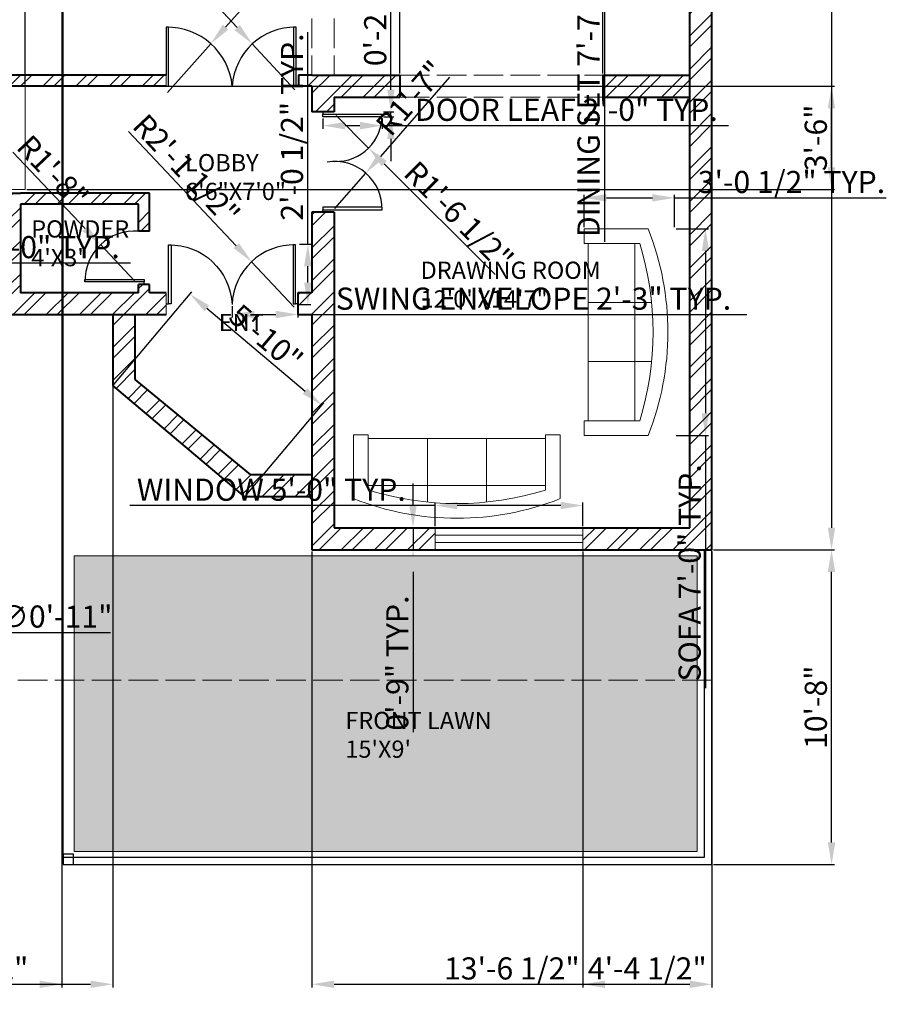
# Model space of a CAD drawing. Units: inches. Extents: x 3815 to 4442, y 1449 to 2534.
# Tile 2 of 5: x 4090 to 4442, y 1449 to 1850. Entities that reach past the tile are written whole.
import ezdxf

# ---------------------------------------------------------------- set-up
doc = ezdxf.new("R2010")
doc.units = ezdxf.units.IN
doc.linetypes.add('ACAD_ISO02W100', pattern=[15, 12, -3])
for name, color, linetype, lineweight in [('A-ANNO-DIMS', 2, 'Continuous', 18), ('A-AREA-IDEN', 7, 'Continuous', 20), ('A-DOOR', 4, 'Continuous', 25), ('A-FLOR-STRS', 7, 'Continuous', 20), ('A-FURN', 8, 'Continuous', 18), ('A-GLAZ', 4, 'Continuous', 20), ('A-ROOF-OVHD', 8, 'ACAD_ISO02W100', 13), ('A-WALL', 7, 'Continuous', 40), ('A-WALL-OVHD', 8, 'ACAD_ISO02W100', 18), ('A-WALL-PATT', 8, 'Continuous', 13), ('C-PROP', 7, 'Continuous', 30), ('L-PLNT', 3, 'Continuous', 18), ('L-PLNT-PATT', 9, 'Continuous', 13)]:
    doc.layers.add(name, color=color, linetype=linetype, lineweight=lineweight)
doc.styles.get("Standard").update_dxf_attribs({"font": 'arial.ttf'})
doc.dimstyles.new('ISO-25', dxfattribs={"dimtxt": 9, "dimasz": 9, "dimexe": 1.25, "dimexo": 0.625, "dimtad": 1, "dimdec": 1, "dimrnd": 9, "dimlunit": 3, "dimtxsty": 'Standard', "dimcen": 2.5, "dimadec": 0, "dimazin": 0, "dimtfac": 1, "dimtdec": 1, "dimtmove": 0, "dimatfit": 3, "dimfxl": 1, "dimarcsym": 0})

# ---------------------------------------------------------------- blocks, each defined once
blk = doc.blocks.new('Sofa - Roundback 7 ft.')
for p, q in [((-12.00002, -32.4421), (-12.00003, -6.5971)), ((11.99997, -32.4421), (11.99998, -6.5971)), ((-36.000027, -34), (-36.000027, -11.4696)), ((35.99998, -34), (35.99998, -11.4696)), ((-35.999844, -13.3819), (35.9998, -13.3819)), ((-36.000027, -32.4421), (35.99998, -32.4421))]:
    blk.add_line(p, q)
for points in [[(-36.000027, -34), (-42.000027, -34), (-42.000027, -8)], [(41.99998, -8), (41.99998, -34), (35.99998, -34)]]:
    blk.add_lwpolyline(points)
for centre, radius, start, end in [((0, -114.25), 114.25, 68.43141, 111.5686), ((-0.00001, -127.1968), 121.1968, 72.72033, 107.2797)]:
    blk.add_arc(centre, radius, start, end)
blk = doc.blocks.new('WIN-W60-9IN')
for p, q in [((0, 9), (0, 0)), ((60, 9), (60, 0)), ((60, 6), (0, 6)), ((60, 3), (0, 3))]:
    blk.add_line(p, q)
blk = doc.blocks.new('DOOR-SWING-24IN')
for p, q in [((25.78, 24.32), (24.78, 24.32)), ((24.78, 24.32), (24.78, 0.32)), ((25.78, 0.32), (25.78, 24.32)), ((24.78, 0.32), (25.78, 0.32)), ((26.78, 0.32), (25.78, 0.32))]:
    blk.add_line(p, q)
blk.add_arc((25.28, -0.98), 25.3, 88.8677, 177.7775)
blk = doc.blocks.new('DOOR-LEAF-24IN')
for p, q in [((0, 2), (0, 1)), ((0, 1), (24, 1)), ((0, 0), (0, 1)), ((24, 0), (0, 0)), ((24, 1), (24, 0))]:
    blk.add_line(p, q)
blk = doc.blocks.new('SITE-PIER')
blk.add_lwpolyline([(0, 0), (4.2, 0), (4.2, 4.28), (0, 4.28)], close=True)
blk = doc.blocks.new('*D18')
at = {"layer": 'A-ANNO-DIMS', "color": 0, "lineweight": -2, "transparency": 16777216}
for p, q in [((4356.58, 1764.74), (4369.81, 1764.74)), ((4368.56, 1755.74), (4368.56, 1689.74)), ((4356.58, 1680.74), (4369.81, 1680.74)), ((4368.56, 1680.74), (4368.56, 1577.95))]:
    blk.add_line(p, q, dxfattribs=at)
at = {"layer": 'A-ANNO-DIMS', "color": 0, "lineweight": 100, "transparency": 16777216}
for points in [[(4367.06, 1755.74), (4370.06, 1755.74), (4368.56, 1764.74)], [(4367.06, 1689.74), (4370.06, 1689.74), (4368.56, 1680.74)]]:
    blk.add_solid(points, dxfattribs=at)
at = {"layer": 'Defpoints', "color": 0, "lineweight": 100, "transparency": 16777216}
for p in [(4355.96, 1764.74), (4355.96, 1680.74), (4368.56, 1680.74)]:
    blk.add_point(p, dxfattribs=at)
at = {"layer": 'A-ANNO-DIMS', "color": 0, "transparency": 16777216, "insert": (4363.28, 1624.85), "char_height": 9, "attachment_point": 5, "rotation": 90}
blk.add_mtext('SOFA 7\'-0" TYP.', dxfattribs=at)
blk = doc.blocks.new('*D19')
at = {"layer": 'A-ANNO-DIMS', "color": 0, "lineweight": -2, "transparency": 16777216}
for p, q in [((4319.29, 1765.37), (4319.29, 1778.59)), ((4355.96, 1765.37), (4355.96, 1778.59)), ((4328.29, 1777.34), (4346.96, 1777.34)), ((4355.96, 1777.34), (4442.03, 1777.34))]:
    blk.add_line(p, q, dxfattribs=at)
at = {"layer": 'A-ANNO-DIMS', "color": 0, "lineweight": 100, "transparency": 16777216}
for points in [[(4328.29, 1778.84), (4328.29, 1775.84), (4319.29, 1777.34)], [(4346.96, 1778.84), (4346.96, 1775.84), (4355.96, 1777.34)]]:
    blk.add_solid(points, dxfattribs=at)
at = {"layer": 'Defpoints', "color": 0, "lineweight": 100, "transparency": 16777216}
for p in [(4355.96, 1777.34), (4319.29, 1764.74), (4355.96, 1764.74)]:
    blk.add_point(p, dxfattribs=at)
at = {"layer": 'A-ANNO-DIMS', "color": 0, "transparency": 16777216, "insert": (4403.5, 1782.62), "char_height": 9, "attachment_point": 5}
blk.add_mtext('3\'-0 1/2" TYP.', dxfattribs=at)
blk = doc.blocks.new('*D20')
at = {"layer": 'A-ANNO-DIMS', "color": 0, "lineweight": -2, "transparency": 16777216}
for p, q in [((4213.13, 1809.67), (4213.13, 1805.45)), ((4237.13, 1809.67), (4237.13, 1805.45)), ((4222.13, 1806.7), (4228.13, 1806.7)), ((4237.13, 1806.7), (4377.94, 1806.7))]:
    blk.add_line(p, q, dxfattribs=at)
at = {"layer": 'A-ANNO-DIMS', "color": 0, "lineweight": 100, "transparency": 16777216}
for points in [[(4222.13, 1808.2), (4222.13, 1805.2), (4213.13, 1806.7)], [(4228.13, 1808.2), (4228.13, 1805.2), (4237.13, 1806.7)]]:
    blk.add_solid(points, dxfattribs=at)
at = {"layer": 'Defpoints', "color": 0, "lineweight": 100, "transparency": 16777216}
for p in [(4213.13, 1810.3), (4237.13, 1810.3), (4237.13, 1806.7)]:
    blk.add_point(p, dxfattribs=at)
at = {"layer": 'A-ANNO-DIMS', "color": 0, "transparency": 16777216, "insert": (4312.03, 1811.98), "char_height": 9, "attachment_point": 5}
blk.add_mtext('DOOR LEAF 2\'-0" TYP.', dxfattribs=at)
blk = doc.blocks.new('*D21')
at = {"layer": 'A-ANNO-DIMS', "color": 0, "lineweight": -2, "transparency": 16777216}
for p, q in [((4240.73, 1821.3), (4240.73, 1886.41)), ((4237.75, 1812.3), (4241.98, 1812.3)), ((4237.75, 1810.3), (4241.98, 1810.3)), ((4240.73, 1810.3), (4240.73, 1812.3)), ((4240.73, 1801.3), (4240.73, 1792.3))]:
    blk.add_line(p, q, dxfattribs=at)
at = {"layer": 'A-ANNO-DIMS', "color": 0, "lineweight": 100, "transparency": 16777216}
for points in [[(4239.23, 1821.3), (4242.23, 1821.3), (4240.73, 1812.3)], [(4239.23, 1801.3), (4242.23, 1801.3), (4240.73, 1810.3)]]:
    blk.add_solid(points, dxfattribs=at)
at = {"layer": 'Defpoints', "color": 0, "lineweight": 100, "transparency": 16777216}
for p in [(4237.13, 1812.3), (4237.13, 1810.3), (4240.73, 1812.3)]:
    blk.add_point(p, dxfattribs=at)
at = {"layer": 'A-ANNO-DIMS', "color": 0, "transparency": 16777216, "insert": (4235.51, 1858.35), "char_height": 9, "attachment_point": 5, "rotation": 90}
blk.add_mtext('0\'-2" TYP.', dxfattribs=at)
blk = doc.blocks.new('*D24')
at = {"layer": 'A-ANNO-DIMS', "color": 0, "lineweight": -2, "transparency": 16777216}
for p, q in [((4258.71, 1643.87), (4258.71, 1653.49)), ((4318.71, 1643.87), (4318.71, 1653.49)), ((4258.71, 1652.24), (4134.57, 1652.24)), ((4309.71, 1652.24), (4267.71, 1652.24))]:
    blk.add_line(p, q, dxfattribs=at)
at = {"layer": 'A-ANNO-DIMS', "color": 0, "lineweight": 100, "transparency": 16777216}
for points in [[(4267.71, 1653.74), (4267.71, 1650.74), (4258.71, 1652.24)], [(4309.71, 1653.74), (4309.71, 1650.74), (4318.71, 1652.24)]]:
    blk.add_solid(points, dxfattribs=at)
at = {"layer": 'Defpoints', "color": 0, "lineweight": 100, "transparency": 16777216}
for p in [(4258.71, 1652.24), (4258.71, 1643.24), (4318.71, 1643.24)]:
    blk.add_point(p, dxfattribs=at)
at = {"layer": 'A-ANNO-DIMS', "color": 0, "transparency": 16777216, "insert": (4192.14, 1657.52), "char_height": 9, "attachment_point": 5}
blk.add_mtext('WINDOW 5\'-0" TYP.', dxfattribs=at)
blk = doc.blocks.new('*D25')
at = {"layer": 'A-ANNO-DIMS', "color": 0, "lineweight": -2, "transparency": 16777216}
for p, q in [((4249.71, 1652.24), (4249.71, 1661.24)), ((4258.08, 1643.24), (4248.46, 1643.24)), ((4249.71, 1643.24), (4249.71, 1634.24)), ((4258.08, 1634.24), (4248.46, 1634.24)), ((4249.71, 1625.24), (4249.71, 1560.13))]:
    blk.add_line(p, q, dxfattribs=at)
at = {"layer": 'A-ANNO-DIMS', "color": 0, "lineweight": 100, "transparency": 16777216}
for points in [[(4248.21, 1652.24), (4251.21, 1652.24), (4249.71, 1643.24)], [(4248.21, 1625.24), (4251.21, 1625.24), (4249.71, 1634.24)]]:
    blk.add_solid(points, dxfattribs=at)
at = {"layer": 'Defpoints', "color": 0, "lineweight": 100, "transparency": 16777216}
for p in [(4258.71, 1643.24), (4249.71, 1634.24), (4258.71, 1634.24)]:
    blk.add_point(p, dxfattribs=at)
at = {"layer": 'A-ANNO-DIMS', "color": 0, "transparency": 16777216, "insert": (4244.49, 1588.19), "char_height": 9, "attachment_point": 5, "rotation": 90}
blk.add_mtext('0\'-9" TYP.', dxfattribs=at)
blk = doc.blocks.new('*D28')
at = {"layer": 'A-ANNO-DIMS', "color": 0, "lineweight": -2, "transparency": 16777216}
for p, q in [((3958.12, 1746.08), (3958.12, 1752.11)), ((3967.12, 1750.86), (3985.12, 1750.86)), ((3994.12, 1746.08), (3994.12, 1752.11)), ((3994.12, 1750.86), (4134.93, 1750.86))]:
    blk.add_line(p, q, dxfattribs=at)
at = {"layer": 'A-ANNO-DIMS', "color": 0, "lineweight": 100, "transparency": 16777216}
for points in [[(3967.12, 1752.36), (3967.12, 1749.36), (3958.12, 1750.86)], [(3985.12, 1752.36), (3985.12, 1749.36), (3994.12, 1750.86)]]:
    blk.add_solid(points, dxfattribs=at)
at = {"layer": 'Defpoints', "color": 0, "lineweight": 100, "transparency": 16777216}
for p in [(3994.12, 1750.86), (3958.12, 1745.46), (3994.12, 1745.46)]:
    blk.add_point(p, dxfattribs=at)
at = {"layer": 'A-ANNO-DIMS', "color": 0, "transparency": 16777216, "insert": (4069.03, 1756.14), "char_height": 9, "attachment_point": 5}
blk.add_mtext('DOOR LEAF 3\'-0" TYP.', dxfattribs=at)
blk = doc.blocks.new('*D38')
at = {"layer": 'A-ANNO-DIMS', "color": 0, "lineweight": -2, "transparency": 16777216}
for p, q in [((4176.16, 1733.3), (4176.16, 1728.66)), ((4185.16, 1729.91), (4193.94, 1729.91)), ((4202.94, 1733.3), (4202.94, 1728.66)), ((4202.94, 1729.91), (4385.39, 1729.91))]:
    blk.add_line(p, q, dxfattribs=at)
at = {"layer": 'A-ANNO-DIMS', "color": 0, "lineweight": 100, "transparency": 16777216}
for points in [[(4185.16, 1731.41), (4185.16, 1728.41), (4176.16, 1729.91)], [(4193.94, 1731.41), (4193.94, 1728.41), (4202.94, 1729.91)]]:
    blk.add_solid(points, dxfattribs=at)
at = {"layer": 'Defpoints', "color": 0, "lineweight": 100, "transparency": 16777216}
for p in [(4176.16, 1733.92), (4202.94, 1733.92), (4202.94, 1729.91)]:
    blk.add_point(p, dxfattribs=at)
at = {"layer": 'A-ANNO-DIMS', "color": 0, "transparency": 16777216, "insert": (4298.67, 1735.19), "char_height": 9, "attachment_point": 5}
blk.add_mtext('SWING ENVELOPE 2\'-3" TYP.', dxfattribs=at)
blk = doc.blocks.new('*D39')
at = {"layer": 'A-ANNO-DIMS', "color": 0, "lineweight": -2, "transparency": 16777216}
for p, q in [((4206.96, 1758.51), (4206.96, 1844.75)), ((4203.57, 1758.51), (4208.21, 1758.51)), ((4206.96, 1742.92), (4206.96, 1749.51)), ((4203.57, 1733.92), (4208.21, 1733.92))]:
    blk.add_line(p, q, dxfattribs=at)
at = {"layer": 'A-ANNO-DIMS', "color": 0, "lineweight": 100, "transparency": 16777216}
for points in [[(4205.46, 1749.51), (4208.46, 1749.51), (4206.96, 1758.51)], [(4205.46, 1742.92), (4208.46, 1742.92), (4206.96, 1733.92)]]:
    blk.add_solid(points, dxfattribs=at)
at = {"layer": 'Defpoints', "color": 0, "lineweight": 100, "transparency": 16777216}
for p in [(4202.94, 1758.51), (4206.96, 1758.51), (4202.94, 1733.92)]:
    blk.add_point(p, dxfattribs=at)
at = {"layer": 'A-ANNO-DIMS', "color": 0, "transparency": 16777216, "insert": (4201.68, 1806.13), "char_height": 9, "attachment_point": 5, "rotation": 90}
blk.add_mtext('2\'-0 1/2" TYP.', dxfattribs=at)
blk = doc.blocks.new('*D46')
at = {"layer": 'A-ANNO-DIMS', "color": 0, "lineweight": -2, "transparency": 16777216}
for p, q in [((4314.45, 1959.69), (4328.73, 1959.69)), ((4327.48, 1950.69), (4327.48, 1877.69)), ((4314.45, 1868.69), (4328.73, 1868.69)), ((4327.48, 1868.69), (4327.48, 1759.52))]:
    blk.add_line(p, q, dxfattribs=at)
at = {"layer": 'A-ANNO-DIMS', "color": 0, "lineweight": 100, "transparency": 16777216}
for points in [[(4325.98, 1950.69), (4328.98, 1950.69), (4327.48, 1959.69)], [(4325.98, 1877.69), (4328.98, 1877.69), (4327.48, 1868.69)]]:
    blk.add_solid(points, dxfattribs=at)
at = {"layer": 'Defpoints', "color": 0, "lineweight": 100, "transparency": 16777216}
for p in [(4313.83, 1959.69), (4313.83, 1868.69), (4327.48, 1868.69)]:
    blk.add_point(p, dxfattribs=at)
at = {"layer": 'A-ANNO-DIMS', "color": 0, "transparency": 16777216, "insert": (4322.2, 1809.6), "char_height": 9, "attachment_point": 5, "rotation": 90}
blk.add_mtext('DINING SET 7\'-7"', dxfattribs=at)
blk = doc.blocks.new('*D51')
at = {"layer": 'A-ANNO-DIMS', "color": 0, "lineweight": -2, "transparency": 16777216}
for p, q in [((4371.75, 1634.24), (4421.03, 1634.24)), ((4419.78, 1515.24), (4419.78, 1625.24)), ((4371.75, 1506.24), (4421.03, 1506.24))]:
    blk.add_line(p, q, dxfattribs=at)
at = {"layer": 'A-ANNO-DIMS', "color": 0, "lineweight": 100, "transparency": 16777216}
for points in [[(4418.28, 1625.24), (4421.28, 1625.24), (4419.78, 1634.24)], [(4418.28, 1515.24), (4421.28, 1515.24), (4419.78, 1506.24)]]:
    blk.add_solid(points, dxfattribs=at)
at = {"layer": 'Defpoints', "color": 0, "lineweight": 100, "transparency": 16777216}
for p in [(4371.13, 1634.24), (4419.78, 1634.24), (4371.13, 1506.24)]:
    blk.add_point(p, dxfattribs=at)
at = {"layer": 'A-ANNO-DIMS', "color": 0, "transparency": 16777216, "insert": (4414.56, 1570.24), "char_height": 9, "attachment_point": 5, "rotation": 90}
blk.add_mtext('10\'-8"', dxfattribs=at)
blk = doc.blocks.new('*D52')
at = {"layer": 'A-ANNO-DIMS', "color": 0, "lineweight": -2, "transparency": 16777216}
for p, q in [((4371.75, 2346.24), (4421.03, 2346.24)), ((4419.78, 2337.24), (4419.78, 1643.24)), ((4371.75, 1634.24), (4421.03, 1634.24))]:
    blk.add_line(p, q, dxfattribs=at)
at = {"layer": 'A-ANNO-DIMS', "color": 0, "lineweight": 100, "transparency": 16777216}
for points in [[(4418.28, 2337.24), (4421.28, 2337.24), (4419.78, 2346.24)], [(4418.28, 1643.24), (4421.28, 1643.24), (4419.78, 1634.24)]]:
    blk.add_solid(points, dxfattribs=at)
at = {"layer": 'Defpoints', "color": 0, "lineweight": 100, "transparency": 16777216}
for p in [(4371.13, 2346.24), (4371.13, 1634.24), (4419.78, 1634.24)]:
    blk.add_point(p, dxfattribs=at)
at = {"layer": 'A-ANNO-DIMS', "color": 0, "transparency": 16777216, "insert": (4414.56, 1990.24), "char_height": 9, "attachment_point": 5, "rotation": 90}
blk.add_mtext('59\'-4"', dxfattribs=at)
blk = doc.blocks.new('*D54')
at = {"layer": 'A-ANNO-DIMS', "color": 0, "lineweight": -2, "transparency": 16777216}
for p, q in [((3996.13, 1823.37), (3996.13, 2516.14)), ((4005.13, 2514.89), (4083.13, 2514.89)), ((4092.13, 1823.37), (4092.13, 2516.14))]:
    blk.add_line(p, q, dxfattribs=at)
at = {"layer": 'A-ANNO-DIMS', "color": 0, "lineweight": 100, "transparency": 16777216}
for points in [[(4005.13, 2516.39), (4005.13, 2513.39), (3996.13, 2514.89)], [(4083.13, 2516.39), (4083.13, 2513.39), (4092.13, 2514.89)]]:
    blk.add_solid(points, dxfattribs=at)
at = {"layer": 'Defpoints', "color": 0, "lineweight": 100, "transparency": 16777216}
for p in [(4092.13, 2514.89), (3996.13, 1822.74), (4092.13, 1822.74)]:
    blk.add_point(p, dxfattribs=at)
at = {"layer": 'A-ANNO-DIMS', "color": 0, "transparency": 16777216, "insert": (4044.13, 2520.11), "char_height": 9, "attachment_point": 5}
blk.add_mtext('8\'-0"', dxfattribs=at)
blk = doc.blocks.new('*D62')
at = {"layer": 'A-ANNO-DIMS', "color": 0, "lineweight": -2, "transparency": 16777216}
for p, q in [((4318.71, 1633.62), (4318.71, 1456.34)), ((4371.13, 1633.62), (4371.13, 1456.34)), ((4327.71, 1457.59), (4362.13, 1457.59))]:
    blk.add_line(p, q, dxfattribs=at)
at = {"layer": 'A-ANNO-DIMS', "color": 0, "lineweight": 100, "transparency": 16777216}
for points in [[(4327.71, 1459.09), (4327.71, 1456.09), (4318.71, 1457.59)], [(4362.13, 1459.09), (4362.13, 1456.09), (4371.13, 1457.59)]]:
    blk.add_solid(points, dxfattribs=at)
at = {"layer": 'Defpoints', "color": 0, "lineweight": 100, "transparency": 16777216}
for p in [(4318.71, 1634.24), (4371.13, 1634.24), (4371.13, 1457.59)]:
    blk.add_point(p, dxfattribs=at)
at = {"layer": 'A-ANNO-DIMS', "color": 0, "transparency": 16777216, "insert": (4344.92, 1462.87), "char_height": 9, "attachment_point": 5}
blk.add_mtext('4\'-4 1/2"', dxfattribs=at)
blk = doc.blocks.new('*D63')
at = {"layer": 'A-ANNO-DIMS', "color": 0, "lineweight": -2, "transparency": 16777216}
for p, q in [((3895.33, 1506.87), (3895.33, 2516.14)), ((3904.33, 2514.89), (4098.56, 2514.89)), ((4107.56, 1506.87), (4107.56, 2516.14))]:
    blk.add_line(p, q, dxfattribs=at)
at = {"layer": 'A-ANNO-DIMS', "color": 0, "lineweight": 100, "transparency": 16777216}
for points in [[(3904.33, 2516.39), (3904.33, 2513.39), (3895.33, 2514.89)], [(4098.56, 2516.39), (4098.56, 2513.39), (4107.56, 2514.89)]]:
    blk.add_solid(points, dxfattribs=at)
at = {"layer": 'Defpoints', "color": 0, "lineweight": 100, "transparency": 16777216}
for p in [(4107.56, 2514.89), (3895.33, 1506.24), (4107.56, 1506.24)]:
    blk.add_point(p, dxfattribs=at)
at = {"layer": 'A-ANNO-DIMS', "color": 0, "transparency": 16777216, "insert": (4001.45, 2520.11), "char_height": 9, "attachment_point": 5}
blk.add_mtext('17\'-8"', dxfattribs=at)
blk = doc.blocks.new('*D66')
at = {"layer": 'A-ANNO-DIMS', "color": 0, "lineweight": -2, "transparency": 16777216}
for p, q in [((4024.63, 2089.28), (4024.63, 1456.34)), ((4107.04, 2089.28), (4107.04, 1456.34)), ((4033.63, 1457.59), (4098.04, 1457.59))]:
    blk.add_line(p, q, dxfattribs=at)
at = {"layer": 'A-ANNO-DIMS', "color": 0, "lineweight": 100, "transparency": 16777216}
for points in [[(4033.63, 1459.09), (4033.63, 1456.09), (4024.63, 1457.59)], [(4098.04, 1459.09), (4098.04, 1456.09), (4107.04, 1457.59)]]:
    blk.add_solid(points, dxfattribs=at)
at = {"layer": 'Defpoints', "color": 0, "lineweight": 100, "transparency": 16777216}
for p in [(4024.63, 2089.9), (4107.04, 2089.9), (4107.04, 1457.59)]:
    blk.add_point(p, dxfattribs=at)
at = {"layer": 'A-ANNO-DIMS', "color": 0, "transparency": 16777216, "insert": (4065.83, 1462.87), "char_height": 9, "attachment_point": 5}
blk.add_mtext('6\'-10 1/2"', dxfattribs=at)
blk = doc.blocks.new('*D70')
at = {"layer": 'A-ANNO-DIMS', "color": 0, "lineweight": -2, "transparency": 16777216}
for p, q in [((4092.75, 1822.74), (4421.03, 1822.74)), ((4419.78, 1789.74), (4419.78, 1813.74)), ((4092.75, 1780.74), (4421.03, 1780.74))]:
    blk.add_line(p, q, dxfattribs=at)
at = {"layer": 'A-ANNO-DIMS', "color": 0, "lineweight": 100, "transparency": 16777216}
for points in [[(4418.28, 1813.74), (4421.28, 1813.74), (4419.78, 1822.74)], [(4418.28, 1789.74), (4421.28, 1789.74), (4419.78, 1780.74)]]:
    blk.add_solid(points, dxfattribs=at)
at = {"layer": 'Defpoints', "color": 0, "lineweight": 100, "transparency": 16777216}
for p in [(4092.13, 1822.74), (4419.78, 1822.74), (4092.13, 1780.74)]:
    blk.add_point(p, dxfattribs=at)
at = {"layer": 'A-ANNO-DIMS', "color": 0, "transparency": 16777216, "insert": (4414.55, 1801.74), "char_height": 9, "attachment_point": 5, "rotation": 90}
blk.add_mtext('3\'-6"', dxfattribs=at)
blk = doc.blocks.new('*D71')
at = {"layer": 'A-ANNO-DIMS', "color": 0, "lineweight": -2, "transparency": 16777216}
for p, q in [((4128.1, 1701.5), (4159.85, 1739.18)), ((4165.93, 1732.43), (4205.85, 1698.8)), ((4181.78, 1656.27), (4213.53, 1693.95))]:
    blk.add_line(p, q, dxfattribs=at)
at = {"layer": 'A-ANNO-DIMS', "color": 0, "lineweight": 100, "transparency": 16777216}
for points in [[(4166.89, 1733.58), (4164.96, 1731.28), (4159.04, 1738.23)], [(4206.81, 1699.94), (4204.88, 1697.65), (4212.73, 1693)]]:
    blk.add_solid(points, dxfattribs=at)
at = {"layer": 'Defpoints', "color": 0, "lineweight": 100, "transparency": 16777216}
for p in [(4127.7, 1701.02), (4212.73, 1693), (4181.38, 1655.79)]:
    blk.add_point(p, dxfattribs=at)
at = {"layer": 'A-ANNO-DIMS', "color": 0, "transparency": 16777216, "insert": (4189.25, 1719.6), "char_height": 9, "attachment_point": 5, "rotation": 319.8858}
blk.add_mtext('5\'-10"', dxfattribs=at)
blk = doc.blocks.new('*D74')
at = {"layer": 'A-ANNO-DIMS', "color": 0, "lineweight": -2, "transparency": 16777216}
for p, q in [((3951.13, 1729.12), (3951.13, 1456.34)), ((4127.7, 1729.12), (4127.7, 1456.34)), ((3960.13, 1457.59), (4118.7, 1457.59))]:
    blk.add_line(p, q, dxfattribs=at)
at = {"layer": 'A-ANNO-DIMS', "color": 0, "lineweight": 100, "transparency": 16777216}
for points in [[(3960.13, 1459.09), (3960.13, 1456.09), (3951.13, 1457.59)], [(4118.7, 1459.09), (4118.7, 1456.09), (4127.7, 1457.59)]]:
    blk.add_solid(points, dxfattribs=at)
at = {"layer": 'Defpoints', "color": 0, "lineweight": 100, "transparency": 16777216}
for p in [(3951.13, 1729.74), (4127.7, 1729.74), (4127.7, 1457.59)]:
    blk.add_point(p, dxfattribs=at)
at = {"layer": 'A-ANNO-DIMS', "color": 0, "transparency": 16777216, "insert": (4039.41, 1462.87), "char_height": 9, "attachment_point": 5}
blk.add_mtext('14\'-8 1/2"', dxfattribs=at)
blk = doc.blocks.new('*D75')
at = {"layer": 'A-ANNO-DIMS', "color": 0, "lineweight": -2, "transparency": 16777216}
for p, q in [((4208.63, 1633.62), (4208.63, 1456.34)), ((4371.13, 1633.62), (4371.13, 1456.34)), ((4217.63, 1457.59), (4362.13, 1457.59))]:
    blk.add_line(p, q, dxfattribs=at)
at = {"layer": 'A-ANNO-DIMS', "color": 0, "lineweight": 100, "transparency": 16777216}
for points in [[(4217.63, 1459.09), (4217.63, 1456.09), (4208.63, 1457.59)], [(4362.13, 1459.09), (4362.13, 1456.09), (4371.13, 1457.59)]]:
    blk.add_solid(points, dxfattribs=at)
at = {"layer": 'Defpoints', "color": 0, "lineweight": 100, "transparency": 16777216}
for p in [(4208.63, 1634.24), (4371.13, 1634.24), (4371.13, 1457.59)]:
    blk.add_point(p, dxfattribs=at)
at = {"layer": 'A-ANNO-DIMS', "color": 0, "transparency": 16777216, "insert": (4289.88, 1462.87), "char_height": 9, "attachment_point": 5}
blk.add_mtext('13\'-6 1/2"', dxfattribs=at)
blk = doc.blocks.new('*D76')
at = {"layer": 'A-ANNO-DIMS', "color": 0, "lineweight": -2, "transparency": 16777216}
for p, q in [((4244.38, 1827.87), (4244.38, 2516.14)), ((4253.38, 2514.89), (4317.89, 2514.89)), ((4326.89, 1827.87), (4326.89, 2516.14))]:
    blk.add_line(p, q, dxfattribs=at)
at = {"layer": 'A-ANNO-DIMS', "color": 0, "lineweight": 100, "transparency": 16777216}
for points in [[(4253.38, 2516.39), (4253.38, 2513.39), (4244.38, 2514.89)], [(4317.89, 2516.39), (4317.89, 2513.39), (4326.89, 2514.89)]]:
    blk.add_solid(points, dxfattribs=at)
at = {"layer": 'Defpoints', "color": 0, "lineweight": 100, "transparency": 16777216}
for p in [(4326.89, 2514.89), (4244.38, 1827.24), (4326.89, 1827.24)]:
    blk.add_point(p, dxfattribs=at)
at = {"layer": 'A-ANNO-DIMS', "color": 0, "transparency": 16777216, "insert": (4285.63, 2520.17), "char_height": 9, "attachment_point": 5}
blk.add_mtext('6\'-10 1/2"', dxfattribs=at)
blk = doc.blocks.new('*D82')
at = {"layer": 'A-ANNO-DIMS', "color": 0, "lineweight": -2, "transparency": 16777216}
for p, q in [((4027.54, 1600.56), (4018.54, 1600.57)), ((4036.54, 1600.55), (4047.56, 1600.53)), ((4126.74, 1600.43), (4056.56, 1600.52))]:
    blk.add_line(p, q, dxfattribs=at)
at = {"layer": 'A-ANNO-DIMS', "color": 0, "lineweight": 100, "transparency": 16777216}
for points in [[(4027.54, 1602.06), (4027.54, 1599.06), (4036.54, 1600.55)], [(4056.56, 1602.02), (4056.56, 1599.02), (4047.56, 1600.53)]]:
    blk.add_solid(points, dxfattribs=at)
at = {"layer": 'Defpoints', "color": 0, "lineweight": 100, "transparency": 16777216}
for p in [(4036.54, 1600.55), (4047.56, 1600.53)]:
    blk.add_point(p, dxfattribs=at)
at = {"layer": 'A-ANNO-DIMS', "color": 0, "transparency": 16777216, "insert": (4096.16, 1605.94), "char_height": 9, "attachment_point": 5, "rotation": 359.927}
blk.add_mtext('4X ∅0\'-11"', dxfattribs=at)
blk = doc.blocks.new('*D86')
at = {"layer": 'A-ANNO-DIMS', "color": 0, "lineweight": -2, "transparency": 16777216}
for p, q in [((4087.06, 1795.89), (4116.5, 1764.84)), ((4136.58, 1743.66), (4122.7, 1758.31))]:
    blk.add_line(p, q, dxfattribs=at)
at = {"layer": 'A-ANNO-DIMS', "color": 0, "lineweight": 100, "transparency": 16777216}
blk.add_solid([(4117.59, 1765.87), (4115.42, 1763.81), (4122.7, 1758.31)], dxfattribs=at)
at = {"layer": 'Defpoints', "color": 0, "lineweight": 100, "transparency": 16777216}
for p in [(4122.7, 1758.31), (4136.58, 1743.66)]:
    blk.add_point(p, dxfattribs=at)
at = {"layer": 'A-ANNO-DIMS', "color": 0, "transparency": 16777216, "insert": (4102.48, 1787.22), "char_height": 9, "attachment_point": 5, "rotation": 313.4752}
blk.add_mtext('R1\'-8"', dxfattribs=at)
blk = doc.blocks.new('*D87')
at = {"layer": 'A-ANNO-DIMS', "color": 0, "lineweight": -2, "transparency": 16777216}
for p, q in [((4218.47, 1810.8), (4231.67, 1797.6)), ((4283.12, 1746.15), (4238.03, 1791.24))]:
    blk.add_line(p, q, dxfattribs=at)
at = {"layer": 'A-ANNO-DIMS', "color": 0, "lineweight": 100, "transparency": 16777216}
blk.add_solid([(4239.09, 1792.3), (4236.97, 1790.18), (4231.67, 1797.6)], dxfattribs=at)
at = {"layer": 'Defpoints', "color": 0, "lineweight": 100, "transparency": 16777216}
for p in [(4218.47, 1810.8), (4231.67, 1797.6)]:
    blk.add_point(p, dxfattribs=at)
at = {"layer": 'A-ANNO-DIMS', "color": 0, "transparency": 16777216, "insert": (4267.49, 1769.25), "char_height": 9, "attachment_point": 5, "rotation": 314.9989}
blk.add_mtext('R1\'-6 1/2"', dxfattribs=at)
blk = doc.blocks.new('*D88')
at = {"layer": 'A-ANNO-DIMS', "color": 0, "lineweight": -2, "transparency": 16777216}
for p, q in [((4264.59, 1826.47), (4236.48, 1794.21)), ((4217.97, 1772.99), (4230.56, 1787.43))]:
    blk.add_line(p, q, dxfattribs=at)
at = {"layer": 'A-ANNO-DIMS', "color": 0, "lineweight": 100, "transparency": 16777216}
blk.add_solid([(4235.35, 1795.2), (4237.61, 1793.23), (4230.56, 1787.43)], dxfattribs=at)
at = {"layer": 'Defpoints', "color": 0, "lineweight": 100, "transparency": 16777216}
for p in [(4230.56, 1787.43), (4217.97, 1772.99)]:
    blk.add_point(p, dxfattribs=at)
at = {"layer": 'A-ANNO-DIMS', "color": 0, "transparency": 16777216, "insert": (4249.61, 1817.11), "char_height": 9, "attachment_point": 5, "rotation": 48.9234}
blk.add_mtext('R1\'-7"', dxfattribs=at)
blk = doc.blocks.new('*D89')
at = {"layer": 'A-ANNO-DIMS', "color": 0, "lineweight": -2, "transparency": 16777216}
for p, q in [((4134.16, 1804.28), (4177.91, 1757.9)), ((4201.44, 1732.94), (4184.08, 1751.35))]:
    blk.add_line(p, q, dxfattribs=at)
at = {"layer": 'A-ANNO-DIMS', "color": 0, "lineweight": 100, "transparency": 16777216}
blk.add_solid([(4179, 1758.93), (4176.82, 1756.87), (4184.08, 1751.35)], dxfattribs=at)
at = {"layer": 'Defpoints', "color": 0, "lineweight": 100, "transparency": 16777216}
for p in [(4184.08, 1751.35), (4201.44, 1732.94)]:
    blk.add_point(p, dxfattribs=at)
at = {"layer": 'A-ANNO-DIMS', "color": 0, "transparency": 16777216, "insert": (4156.79, 1787.99), "char_height": 9, "attachment_point": 5, "rotation": 313.3224}
blk.add_mtext('R2\'-1 1/2"', dxfattribs=at)
blk = doc.blocks.new('*D90')
at = {"layer": 'A-ANNO-DIMS', "color": 0, "lineweight": -2, "transparency": 16777216}
for p, q in [((4215.97, 1894.31), (4173.53, 1846.73)), ((4149.88, 1820.22), (4167.53, 1840.01))]:
    blk.add_line(p, q, dxfattribs=at)
at = {"layer": 'A-ANNO-DIMS', "color": 0, "lineweight": 100, "transparency": 16777216}
blk.add_solid([(4172.41, 1847.73), (4174.65, 1845.73), (4167.53, 1840.01)], dxfattribs=at)
at = {"layer": 'Defpoints', "color": 0, "lineweight": 100, "transparency": 16777216}
for p in [(4167.53, 1840.01), (4149.88, 1820.22)]:
    blk.add_point(p, dxfattribs=at)
at = {"layer": 'A-ANNO-DIMS', "color": 0, "transparency": 16777216, "insert": (4193.8, 1877.39), "char_height": 9, "attachment_point": 5, "rotation": 48.2637}
blk.add_mtext('R2\'-2 1/2"', dxfattribs=at)
blk = doc.blocks.new('*D91')
at = {"layer": 'A-ANNO-DIMS', "color": 0, "lineweight": -2, "transparency": 16777216}
for p, q in [((4134.94, 1893.34), (4178.27, 1846.57)), ((4201.68, 1821.3), (4184.39, 1839.97))]:
    blk.add_line(p, q, dxfattribs=at)
at = {"layer": 'A-ANNO-DIMS', "color": 0, "lineweight": 100, "transparency": 16777216}
blk.add_solid([(4179.37, 1847.59), (4177.17, 1845.55), (4184.39, 1839.97)], dxfattribs=at)
at = {"layer": 'Defpoints', "color": 0, "lineweight": 100, "transparency": 16777216}
for p in [(4184.39, 1839.97), (4201.68, 1821.3)]:
    blk.add_point(p, dxfattribs=at)
at = {"layer": 'A-ANNO-DIMS', "color": 0, "transparency": 16777216, "insert": (4157.42, 1876.84), "char_height": 9, "attachment_point": 5, "rotation": 312.817}
blk.add_mtext('R2\'-1 1/2"', dxfattribs=at)

msp = doc.modelspace()

# ---------------------------------------------------------------- hatches: boundary and pattern name
at = {"layer": 'A-WALL-PATT'}
h = msp.add_hatch(dxfattribs=at)
h.set_pattern_fill('ANSI32', color=256)
h.paths.add_polyline_path([(4156.29, 2346.24), (3989.15, 2346.24), (3989.15, 2337.24), (4044.13, 2337.24), (4044.13, 2305.59, -0.025534), (4046.38, 2305.51), (4048.63, 2305.51), (4048.63, 2337.24), (4139.63, 2337.24), (4139.63, 2277.24), (4112.45, 2277.24), (4112.45, 2272.74), (4139.63, 2272.74), (4139.63, 2180.66), (4148.63, 2180.66), (4148.63, 2184.24), (4208.63, 2184.24), (4208.63, 2180.66), (4213.13, 2180.66), (4213.13, 2209.79), (4208.63, 2209.79), (4208.63, 2188.74), (4148.63, 2188.74), (4148.63, 2254.74), (4185.97, 2254.74), (4185.97, 2259.24), (4148.63, 2259.24), (4148.63, 2337.24), (4156.29, 2337.24)])
h.paths.add_polyline_path([(4251.85, 2346.24), (4180.29, 2346.24), (4180.29, 2337.24), (4208.63, 2337.24), (4208.63, 2259.24), (4205.62, 2259.24), (4205.62, 2254.74), (4208.63, 2254.74), (4208.63, 2245.05), (4213.13, 2245.05), (4213.13, 2337.24), (4251.85, 2337.24)])
h.paths.add_polyline_path([(4371.13, 2346.24), (4311.85, 2346.24), (4311.85, 2337.24), (4362.13, 2337.24), (4362.13, 2129.24), (4213.13, 2129.24), (4213.13, 2137.97), (4208.63, 2137.97), (4208.63, 2111.87), (4217.63, 2111.87), (4217.63, 2120.24), (4362.13, 2120.24), (4362.13, 1643.24), (4318.71, 1643.24), (4318.71, 1634.24), (4371.13, 1634.24)])
h.paths.add_polyline_path([(3960.13, 2175.52), (3951.13, 2175.52), (3951.13, 2089.9), (3960.13, 2089.9), (3960.13, 2120.24), (4020.13, 2120.24), (4020.13, 2084.42), (4024.63, 2084.42), (4024.63, 2120.24), (4139.63, 2120.24), (4139.63, 2062.37), (4148.63, 2062.37), (4148.63, 2137.97), (4139.63, 2137.97), (4139.63, 2129.24), (3960.13, 2129.24)])
h.paths.add_polyline_path([(3960.13, 2272.74), (4044.13, 2272.74), (4079.8, 2272.74), (4079.8, 2277.24), (4048.63, 2277.24), (4048.63, 2282.04), (4044.13, 2282.04), (4044.13, 2277.24), (3960.13, 2277.24), (3960.13, 2337.24), (3965.15, 2337.24), (3965.15, 2346.24), (3951.13, 2346.24), (3951.13, 2235.52), (3960.13, 2235.52)])
h.paths.add_polyline_path([(4024.63, 2050.34), (4020.13, 2050.34), (4020.13, 2012.24), (3960.13, 2012.24), (3960.13, 2051.05), (3951.13, 2051.05), (3951.13, 1979.78), (3960.13, 1979.78), (3960.13, 2003.24), (4024.63, 2003.24)])
h.paths.add_polyline_path([(4217.63, 2072.24), (4208.63, 2072.24), (4208.63, 2015.24), (4362.13, 2015.24), (4362.13, 2024.24), (4217.63, 2024.24)], flags=17)
h.paths.add_polyline_path([(3960.13, 1940.92), (3951.13, 1940.92), (3951.13, 1883.13), (3960.13, 1883.13)])
h.paths.add_polyline_path([(3960.13, 1822.74), (4149.38, 1822.74), (4149.38, 1827.24), (3960.13, 1827.24), (3960.13, 1844.28), (3951.13, 1844.28), (3951.13, 1769.4), (3960.13, 1769.4)])
h.paths.add_polyline_path([(4362.13, 1827.24), (4326.89, 1827.24), (4326.89, 1818.24), (4362.13, 1818.24)], flags=17)
h.paths.add_polyline_path([(4244.38, 1827.24), (4208.63, 1827.24), (4203.18, 1827.24), (4203.18, 1822.74), (4208.63, 1822.74), (4208.63, 1812.3), (4217.63, 1812.3), (4217.63, 1818.24), (4244.38, 1818.24)])
h.paths.add_polyline_path([(4149.38, 1738.74), (4142.66, 1738.74), (4142.66, 1742.16), (4138.16, 1742.16), (4138.16, 1738.74), (4090.16, 1738.74), (4090.16, 1774.74), (4138.16, 1774.74), (4138.16, 1763.78), (4142.66, 1763.78), (4142.66, 1774.74), (4142.66, 1779.24), (4138.16, 1779.24), (4090.16, 1779.24), (4085.66, 1779.24), (4085.66, 1774.74), (4085.66, 1738.74), (3960.13, 1738.74), (3960.13, 1743.46), (3951.13, 1743.46), (3951.13, 1729.74), (4149.38, 1729.74)])
h.paths.add_polyline_path([(4136.7, 1703.49), (4136.7, 1729.74), (4127.7, 1729.74), (4127.7, 1703.49), (4127.7, 1701.02), (4181.38, 1655.79), (4183.63, 1655.79), (4208.63, 1655.79), (4208.63, 1664.79), (4183.63, 1664.79)])
h.paths.add_polyline_path([(4217.63, 1771.49), (4208.63, 1771.49), (4208.63, 1738.74), (4202.94, 1738.74), (4202.94, 1729.74), (4208.63, 1729.74), (4208.63, 1634.24), (4258.71, 1634.24), (4258.71, 1643.24), (4217.63, 1643.24)])
at = {"layer": 'L-PLNT-PATT'}
h = msp.add_hatch(dxfattribs=at)
h.set_pattern_fill('GOST_GLASS', color=256)
h.paths.add_polyline_path([(4368.13, 2463.24), (3894.13, 2463.24, -0.246049), (3960.13, 2346.24), (4368.13, 2346.24)])
h.paths.add_polyline_path([(4365.15, 1631.83), (4112.05, 1631.83), (4112.05, 1581.3), (4365.15, 1581.3)])
h.paths.add_polyline_path([(4365.15, 1581.3), (4112.05, 1581.3), (4112.05, 1511.54), (4365.15, 1511.54)])
h.paths.add_polyline_path([(4219.4, 1545.72), (4287.81, 1545.72), (4287.81, 1571.84), (4219.4, 1571.84)], flags=24)

# ---------------------------------------------------------------- linework, layer by layer
at = {"layer": 'A-DOOR'}
for p, q in [((4150.38, 1846.74), (4149.38, 1846.74)), ((4149.38, 1846.74), (4149.38, 1827.24)), ((4150.38, 1822.74), (4150.38, 1846.74)), ((4202.18, 1846.74), (4201.18, 1846.74)), ((4201.18, 1846.74), (4201.18, 1822.74)), ((4202.18, 1822.74), (4202.18, 1846.74)), ((4149.38, 1822.74), (4150.38, 1822.74)), ((4203.18, 1822.74), (4202.18, 1822.74))]:
    msp.add_line(p, q, dxfattribs=at)
for centre, radius, start, end in [((4149.88, 1820.22), 26.52, 5.4473, 91.0802), ((4201.68, 1821.3), 25.44, 88.874, 176.759), ((4218.47, 1810.8), 18.66, 268.4594, 1.5355), ((4217.97, 1772.99), 19.16, 358.5047, 99.3417), ((4136.58, 1743.66), 20.18, 85.5312, 181.4195)]:
    msp.add_arc(centre, radius, start, end, dxfattribs=at)
at = {"layer": 'A-FLOR-STRS'}
for p in [(4092.13, 1822.74), (3996.13, 1780.74)]:
    msp.add_line(p, (4092.13, 1780.74), dxfattribs=at)
at = {"layer": 'A-ROOF-OVHD'}
msp.add_line((3894.13, 1581.3), (4371.13, 1581.3), dxfattribs=at)
at = {"layer": 'A-WALL'}
for p, q in [((4371.13, 1634.24), (4371.13, 2346.24)), ((4362.13, 1643.24), (4362.13, 2120.24)), ((4149.38, 1827.24), (3960.13, 1827.24)), ((4208.63, 1827.24), (4203.18, 1827.24)), ((4203.18, 1827.24), (4203.18, 1822.74)), ((4208.63, 1827.24), (4244.38, 1827.24)), ((4244.38, 1827.24), (4244.38, 1818.24)), ((4326.89, 1827.24), (4326.89, 1818.24)), ((4326.89, 1827.24), (4362.13, 1827.24)), ((4149.38, 1822.74), (3960.13, 1822.74)), ((4208.63, 1822.74), (4203.18, 1822.74)), ((4208.63, 1822.74), (4208.63, 1812.3)), ((4217.63, 1818.24), (4217.63, 1812.3)), ((4217.63, 1818.24), (4244.38, 1818.24)), ((4217.63, 1818.24), (4217.63, 1812.3)), ((4326.89, 1818.24), (4362.13, 1818.24)), ((4217.63, 1812.3), (4208.63, 1812.3)), ((4085.66, 1779.24), (4090.16, 1779.24)), ((4138.16, 1779.24), (4090.16, 1779.24)), ((4142.66, 1779.24), (4138.16, 1779.24)), ((4142.66, 1774.74), (4142.66, 1779.24)), ((4138.16, 1774.74), (4090.16, 1774.74)), ((4090.16, 1774.74), (4090.16, 1738.74)), ((4138.16, 1763.78), (4138.16, 1774.74)), ((4142.66, 1763.78), (4142.66, 1774.74)), ((4217.63, 1771.49), (4208.63, 1771.49)), ((4208.63, 1771.49), (4208.63, 1738.74)), ((4217.63, 1771.49), (4217.63, 1643.24)), ((4217.63, 1771.49), (4217.63, 1738.74)), ((4142.66, 1763.78), (4138.16, 1763.78)), ((4138.16, 1738.74), (4138.16, 1742.16)), ((4142.66, 1742.16), (4138.16, 1742.16)), ((4142.66, 1738.74), (4142.66, 1742.16)), ((4138.16, 1738.74), (4090.16, 1738.74)), ((4149.38, 1738.74), (4142.66, 1738.74)), ((4208.63, 1738.74), (4202.94, 1738.74)), ((4202.94, 1738.74), (4202.94, 1729.74)), ((4149.38, 1729.74), (3951.13, 1729.74)), ((4127.7, 1729.74), (4127.7, 1703.49)), ((4136.7, 1729.74), (4136.7, 1703.49)), ((4208.63, 1729.74), (4202.94, 1729.74)), ((4208.63, 1729.74), (4208.63, 1634.24)), ((4127.7, 1703.49), (4127.7, 1701.02)), ((4136.7, 1703.49), (4183.63, 1664.79)), ((4181.38, 1655.79), (4127.7, 1701.02)), ((4208.63, 1664.79), (4183.63, 1664.79)), ((4183.63, 1655.79), (4181.38, 1655.79)), ((4208.63, 1655.79), (4183.63, 1655.79)), ((4217.63, 1643.24), (4362.13, 1643.24)), ((4208.63, 1634.24), (4371.13, 1634.24))]:
    msp.add_line(p, q, dxfattribs=at)
at = {"layer": 'A-WALL-OVHD'}
for p, q in [((4208.63, 2015.24), (4208.63, 1827.24)), ((4217.63, 2015.24), (4217.63, 1827.24)), ((4149.38, 1827.24), (4149.38, 1822.74)), ((4244.38, 1827.24), (4326.89, 1827.24)), ((4244.38, 1818.24), (4326.89, 1818.24)), ((4149.38, 1738.74), (4149.38, 1729.74))]:
    msp.add_line(p, q, dxfattribs=at)
at = {"layer": 'C-PROP'}
for p, q in [((4368.13, 1509.24), (4368.13, 1634.24)), ((4371.13, 1506.24), (4371.13, 1634.24)), ((4107.56, 1509.24), (4368.13, 1509.24)), ((4107.56, 1506.24), (4371.13, 1506.24))]:
    msp.add_line(p, q, dxfattribs=at)
at = {"layer": 'L-PLNT'}
for p, q in [((4112.05, 1511.54), (4112.05, 1631.83)), ((4112.05, 1631.83), (4365.15, 1631.83)), ((4365.15, 1631.83), (4365.15, 1511.54)), ((4365.15, 1511.54), (4112.05, 1511.54))]:
    msp.add_line(p, q, dxfattribs=at)

# ---------------------------------------------------------------- block references
at = {"layer": 'A-DOOR'}
for name, p in [('DOOR-LEAF-24IN', (4213.13, 1810.3)), ('DOOR-SWING-24IN', (4176.16, 1733.92))]:
    msp.add_blockref(name, p, dxfattribs=at)
at = {"layer": 'A-DOOR', "extrusion": (0, 0, -1), "zscale": -1, "rotation": 180}
msp.add_blockref('DOOR-LEAF-24IN', (-4213.13, 1773.49), dxfattribs=at)
at = {"layer": 'A-DOOR', "extrusion": (0, 0, -1), "zscale": -1}
msp.add_blockref('DOOR-SWING-24IN', (-4176.16, 1733.92), dxfattribs=at)
at = {"layer": 'A-DOOR', "rotation": 180}
msp.add_blockref('DOOR-LEAF-24IN', (4140.41, 1744.16), dxfattribs=at)
at = {"layer": 'A-FURN'}
for p, rotation in [((4353.29, 1722.74), 270), ((4267.55, 1647.05), 180)]:
    msp.add_blockref('Sofa - Roundback 7 ft.', p, dxfattribs=dict(at, rotation=rotation))
at = {"layer": 'A-GLAZ', "rotation": 180}
msp.add_blockref('WIN-W60-9IN', (4318.71, 1643.24), dxfattribs=at)
at = {"layer": 'C-PROP'}
msp.add_blockref('SITE-PIER', (4107.56, 1506.24), dxfattribs=at)

# ---------------------------------------------------------------- texts
at = {"layer": 'A-AREA-IDEN', "char_height": 7, "attachment_point": 1}
for s, width, insert in [('LOBBY\\P6\'6"X7\'0"', 62.2181, (4157.07, 1795.13)), ("POWDER\\P4'X3'", 62.2181, (4094.57, 1768.21)), ('DRAWING ROOM\\P12\'0"X14\'7"', 126.3434, (4252.79, 1751.4)), ('ENT', 62.2181, (4170.77, 1730.14)), ("FRONT LAWN\\P15'X9'", 95.3196, (4222.22, 1568.36))]:
    msp.add_mtext_dynamic_manual_height_columns(s, width=width, gutter_width=12.5, heights=[0], dxfattribs=dict(at, insert=insert))

# ---------------------------------------------------------------- dimensions: what is measured, and where the dimension line sits
at = {"layer": 'A-ANNO-DIMS'}
for base, p1, p2, picture, middle in [((4326.89, 2514.89), (4244.38, 1827.24), (4326.89, 1827.24), '*D76', (4285.63, 2520.17)), ((4107.56, 2514.89), (3895.33, 1506.24), (4107.56, 1506.24), '*D63', (4001.45, 2520.11)), ((4092.13, 2514.89), (3996.13, 1822.74), (4092.13, 1822.74), '*D54', (4044.13, 2520.11)), ((4107.04, 1457.59), (4024.63, 2089.9), (4107.04, 2089.9), '*D66', (4065.83, 1462.87)), ((4127.7, 1457.59), (3951.13, 1729.74), (4127.7, 1729.74), '*D74', (4039.41, 1462.87)), ((4371.13, 1457.59), (4208.63, 1634.24), (4371.13, 1634.24), '*D75', (4289.88, 1462.87)), ((4371.13, 1457.59), (4318.71, 1634.24), (4371.13, 1634.24), '*D62', (4344.92, 1462.87))]:
    dim = msp.add_linear_dim(base=base, p1=p1, p2=p2, dimstyle='ISO-25', override={"dimdec": 1, "dimlfac": 1, "dimrnd": 0, "dimzin": 1, "dimdsep": 46, "dimlunit": 4, "dimfrac": 2}, dxfattribs=at)
    dim.commit()
    dim.dimension.update_dxf_attribs({"geometry": picture, "text_midpoint": middle})
for base, p1, p2, angle, picture, middle in [((4419.78, 1634.24), (4371.13, 2346.24), (4371.13, 1634.24), 90, '*D52', (4414.56, 1990.24)), ((4419.78, 1822.74), (4092.13, 1780.74), (4092.13, 1822.74), 90, '*D70', (4414.55, 1801.74)), ((4212.73, 1693), (4127.7, 1701.02), (4181.38, 1655.79), 319.8858, '*D71', (4189.25, 1719.6)), ((4419.78, 1634.24), (4371.13, 1506.24), (4371.13, 1634.24), 90, '*D51', (4414.56, 1570.24))]:
    dim = msp.add_linear_dim(base=base, p1=p1, p2=p2, angle=angle, dimstyle='ISO-25', override={"dimdec": 1, "dimlfac": 1, "dimrnd": 0, "dimzin": 1, "dimdsep": 46, "dimlunit": 4, "dimfrac": 2}, dxfattribs=at)
    dim.commit()
    dim.dimension.update_dxf_attribs({"geometry": picture, "text_midpoint": middle})
for base, p1, p2, angle, text, picture, middle in [((4327.48, 1868.69), (4313.83, 1959.69), (4313.83, 1868.69), 270, 'DINING SET <>', '*D46', (4322.2, 1809.6)), ((4240.73, 1812.3), (4237.13, 1810.3), (4237.13, 1812.3), 90, '<> TYP.', '*D21', (4235.51, 1858.35)), ((4206.96, 1758.51), (4202.94, 1733.92), (4202.94, 1758.51), 90, '<> TYP.', '*D39', (4201.68, 1806.13)), ((4368.56, 1680.74), (4355.96, 1764.74), (4355.96, 1680.74), 270, 'SOFA <> TYP.', '*D18', (4363.28, 1624.85)), ((4258.71, 1652.24), (4318.71, 1643.24), (4258.71, 1643.24), 180, 'WINDOW <> TYP.', '*D24', (4192.14, 1657.52)), ((4249.71, 1634.24), (4258.71, 1643.24), (4258.71, 1634.24), 270, '<> TYP.', '*D25', (4244.49, 1588.19))]:
    dim = msp.add_linear_dim(base=base, p1=p1, p2=p2, angle=angle, text=text, dimstyle='ISO-25', override={"dimdec": 1, "dimlfac": 1, "dimrnd": 0, "dimzin": 1, "dimdsep": 46, "dimlunit": 4, "dimfrac": 2}, dxfattribs=at)
    dim.commit()
    dim.dimension.update_dxf_attribs({"geometry": picture, "text_midpoint": middle})
for center, mpoint, picture, middle in [((4149.88, 1820.22), (4167.53, 1840.01), '*D90', (4193.8, 1877.39)), ((4201.68, 1821.3), (4184.39, 1839.97), '*D91', (4157.42, 1876.84)), ((4217.97, 1772.99), (4230.56, 1787.43), '*D88', (4249.61, 1817.11)), ((4201.44, 1732.94), (4184.08, 1751.35), '*D89', (4156.79, 1787.99)), ((4218.47, 1810.8), (4231.67, 1797.6), '*D87', (4267.49, 1769.25)), ((4136.58, 1743.66), (4122.7, 1758.31), '*D86', (4102.48, 1787.22))]:
    dim = msp.add_radius_dim(center=center, mpoint=mpoint, dimstyle='ISO-25', override={"dimdec": 1, "dimlfac": 1, "dimrnd": 0, "dimzin": 1, "dimdsep": 46, "dimlunit": 4, "dimfrac": 2}, dxfattribs=at)
    dim.commit()
    dim.dimension.update_dxf_attribs({"geometry": picture, "text_midpoint": middle})
for base, p1, p2, text, picture, middle in [((4237.13, 1806.7), (4213.13, 1810.3), (4237.13, 1810.3), 'DOOR LEAF <> TYP.', '*D20', (4312.03, 1811.98)), ((4355.96, 1777.34), (4319.29, 1764.74), (4355.96, 1764.74), '<> TYP.', '*D19', (4403.5, 1782.62)), ((3994.12, 1750.86), (3958.12, 1745.46), (3994.12, 1745.46), 'DOOR LEAF <> TYP.', '*D28', (4069.03, 1756.14)), ((4202.94, 1729.91), (4176.16, 1733.92), (4202.94, 1733.92), 'SWING ENVELOPE <> TYP.', '*D38', (4298.67, 1735.19))]:
    dim = msp.add_linear_dim(base=base, p1=p1, p2=p2, text=text, dimstyle='ISO-25', override={"dimdec": 1, "dimlfac": 1, "dimrnd": 0, "dimzin": 1, "dimdsep": 46, "dimlunit": 4, "dimfrac": 2}, dxfattribs=at)
    dim.commit()
    dim.dimension.update_dxf_attribs({"geometry": picture, "text_midpoint": middle})
dim = msp.add_diameter_dim_2p(p1=(4036.54, 1600.55), p2=(4047.56, 1600.53), text='4X <>', dimstyle='ISO-25', override={"dimdec": 1, "dimlfac": 1, "dimrnd": 0, "dimzin": 1, "dimdsep": 46, "dimlunit": 4, "dimfrac": 2}, dxfattribs=at)
dim.commit()
dim.dimension.update_dxf_attribs({"geometry": '*D82', "text_midpoint": (4096.15, 1600.47)})

doc.saveas('drawing.dxf')
